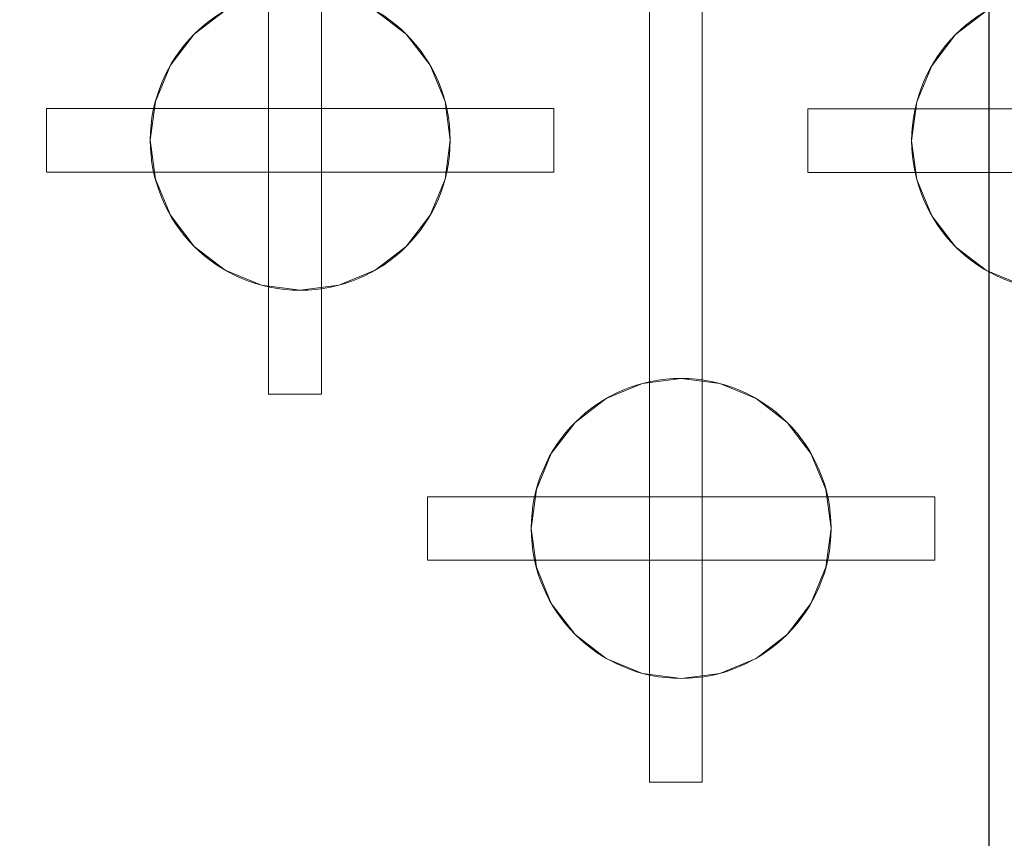
# Model space of a CAD drawing. Units: inches. Extents: x 2696 to 3240, y 1564 to 2310.
# Tile 44 of 76: x 2777.108 to 2782.926, y 2084.368 to 2089.203. Entities that reach past the tile are written whole.
import ezdxf

# ---------------------------------------------------------------- set-up
doc = ezdxf.new("R2010")
doc.units = ezdxf.units.IN
for name, color, linetype, lineweight in [('A-ANNO-DIMS', 3, 'Continuous', 18), ('A-FLOR-FIXT', 8, 'Continuous', 18), ('A-FURN', 251, 'Continuous', 13)]:
    doc.layers.add(name, color=color, linetype=linetype, lineweight=lineweight)
doc.styles.add('TIMES NEW', font='times.ttf')
doc.dimstyles.new('Siddhuu', dxfattribs={"dimtxt": 6, "dimasz": 2.5, "dimexe": 1.25, "dimexo": 0.625, "dimtad": 1, "dimdec": 1, "dimlunit": 4, "dimtxsty": 'TIMES NEW', "dimcen": 2.5, "dimclrd": 256, "dimclre": 1, "dimclrt": 7, "dimadec": 0, "dimazin": 0, "dimtfac": 1, "dimtdec": 1, "dimtmove": 0, "dimatfit": 3, "dimfxl": 1, "dimtolj": 1, "dimlwd": -1, "dimarcsym": 0})

# ---------------------------------------------------------------- blocks, each defined once
blk = doc.blocks.new('A$C1af1f523')
at = {"layer": 'A-FURN'}
for p, q in [((-2.9003, 3.9351), (-2.9003, 0.9365)), ((-2.9003, 3.9351, 0.5), (-2.9003, 0.9365, 0.5)), ((-2.5253, 3.9351), (-2.5253, 0.9365)), ((-2.5253, 3.9351, 0.5), (-2.5253, 0.9365, 0.5)), ((-3.4801, 1.9924), (-3.4801, 1.9924, 0.5)), ((-3.3393, 1.8089), (-3.3393, 1.8089, 0.5)), ((-2.0863, 1.8089), (-2.0863, 1.8089, 0.5)), ((-4.8156, 1.6871), (-5.1906, 1.6871)), ((-4.8156, 1.6871, 0.5), (-5.1906, 1.6871, 0.5)), ((-5.1906, 1.6871), (-5.1906, 1.6871, 0.5)), ((-5.1906, 1.6871), (-5.1901, -1.3115)), ((-5.1906, 1.6871, 0.5), (-5.1901, -1.3115, 0.5)), ((-4.8156, 1.6871), (-4.8156, 1.6871, 0.5)), ((-4.8156, 1.6871), (-4.8151, -1.3115)), ((-4.8156, 1.6871, 0.5), (-4.8151, -1.3115, 0.5)), ((-3.1558, 1.6681), (-3.1558, 1.6681, 0.5)), ((-2.2698, 1.6681), (-2.2698, 1.6681, 0.5)), ((-2.9421, 1.5796), (-2.9421, 1.5796, 0.5)), ((-2.4835, 1.5796), (-2.4835, 1.5796, 0.5)), ((-2.7128, 1.5494), (-2.7128, 1.5494, 0.5)), ((-5.0026, 1.0735), (-5.0026, 1.0735, 0.5)), ((-5.232, 1.0433), (-5.232, 1.0433, 0.5)), ((-4.7733, 1.0433), (-4.7733, 1.0433, 0.5)), ((-5.4457, 0.9548), (-5.4457, 0.9548, 0.5)), ((-4.5596, 0.9548), (-4.5596, 0.9548, 0.5)), ((-2.9003, 0.9365), (-2.9003, 0.9365, 0.5)), ((-2.5253, 0.9365), (-2.8979, 0.9365)), ((-2.5253, 0.9365, 0.5), (-2.8979, 0.9365, 0.5)), ((-2.8979, 0.9365), (-2.8979, 0.9365, 0.5)), ((-2.5253, 0.9365), (-2.5253, 0.9365, 0.5)), ((-5.6292, 0.814), (-5.6292, 0.814, 0.5)), ((-4.3761, 0.814), (-4.3761, 0.814, 0.5)), ((-5.77, 0.6305), (-5.77, 0.6305, 0.5)), ((-4.2353, 0.6305), (-4.2353, 0.6305, 0.5)), ((-5.8585, 0.4168), (-5.8585, 0.4168, 0.5)), ((-4.1468, 0.4168), (-4.1468, 0.4168, 0.5)), ((0, 0.3125), (-6.5015, 0.3125)), ((0, 0.3125, 0.5), (-6.5015, 0.3125, 0.5)), ((-6.5015, 0.3125), (-6.5015, 0.3125, 0.5)), ((-6.5015, 0.3114), (-6.5015, 0)), ((-6.5015, 0.3114, 0.5), (-6.5015, 0, 0.5)), ((-6.5015, 0.3114), (-6.5015, 0.3114, 0.5)), ((-5.8887, 0.1875), (-5.8887, 0.1875, 0.5)), ((-4.1166, 0.1875), (-4.1166, 0.1875, 0.5)), ((0, 0), (-6.5015, 0)), ((0, 0, 0.5), (-6.5015, 0, 0.5)), ((-6.5015, 0), (-6.5015, 0, 0.5)), ((-6.5015, 0), (-6.5015, -0.0011)), ((-6.5015, 0, 0.5), (-6.5015, -0.0011, 0.5)), ((-6.5015, -0.0011), (-6.5015, -0.0011, 0.5)), ((-5.8585, -0.0418), (-5.8585, -0.0418, 0.5)), ((-4.1468, -0.0418), (-4.1468, -0.0418, 0.5)), ((-5.77, -0.2555), (-5.77, -0.2555, 0.5)), ((-4.2353, -0.2555), (-4.2353, -0.2555, 0.5)), ((-5.6292, -0.439), (-5.6292, -0.439, 0.5)), ((-4.3761, -0.439), (-4.3761, -0.439, 0.5)), ((-5.4457, -0.5798), (-5.4457, -0.5798, 0.5)), ((-4.5596, -0.5798), (-4.5596, -0.5798, 0.5)), ((-2.898, -0.5642), (-2.898, -3.5628)), ((-2.898, -0.5642, 0.5), (-2.898, -3.5628, 0.5)), ((-2.898, -0.5642), (-2.898, -0.5642, 0.5)), ((-2.523, -0.5642), (-2.898, -0.5642)), ((-2.523, -0.5642, 0.5), (-2.898, -0.5642, 0.5)), ((-2.523, -0.5642), (-2.523, -3.5628)), ((-2.523, -0.5642, 0.5), (-2.523, -3.5628, 0.5)), ((-2.523, -0.5642), (-2.523, -0.5642, 0.5)), ((-5.232, -0.6683), (-5.232, -0.6683, 0.5)), ((-4.7733, -0.6683), (-4.7733, -0.6683, 0.5)), ((-5.0026, -0.6985), (-5.0026, -0.6985, 0.5)), ((-2.9398, -1.208), (-2.9398, -1.208, 0.5)), ((-2.7105, -1.1778), (-2.7105, -1.1778, 0.5)), ((-2.4812, -1.208), (-2.4812, -1.208, 0.5)), ((-5.1901, -1.3115), (-5.1901, -1.3115, 0.5)), ((-4.8151, -1.3115), (-5.1878, -1.3115)), ((-4.8151, -1.3115, 0.5), (-5.1878, -1.3115, 0.5)), ((-5.1878, -1.3115), (-5.1878, -1.3115, 0.5)), ((-4.8151, -1.3115), (-4.8151, -1.3115, 0.5)), ((-3.1535, -1.2965), (-3.1535, -1.2965, 0.5)), ((-2.2675, -1.2965), (-2.2675, -1.2965, 0.5)), ((-3.337, -1.4373), (-3.337, -1.4373, 0.5)), ((-2.084, -1.4373), (-2.084, -1.4373, 0.5)), ((-3.4778, -1.6208), (-3.4778, -1.6208, 0.5)), ((-3.5664, -1.8345), (-3.5664, -1.8345, 0.5)), ((0, -1.9388), (-4.2094, -1.9388)), ((0, -1.9388, 0.5), (-4.2094, -1.9388, 0.5)), ((-4.2094, -1.9388), (-4.2094, -1.9388, 0.5)), ((-4.2094, -1.9399), (-4.2094, -2.2513)), ((-4.2094, -1.9399, 0.5), (-4.2094, -2.2513, 0.5)), ((-4.2094, -1.9399), (-4.2094, -1.9399, 0.5)), ((-3.5965, -2.0638), (-3.5965, -2.0638, 0.5)), ((0, -2.2513), (-4.2094, -2.2513)), ((0, -2.2513, 0.5), (-4.2094, -2.2513, 0.5)), ((-4.2094, -2.2513), (-4.2094, -2.2513, 0.5)), ((-4.2094, -2.2513), (-4.2094, -2.2524)), ((-4.2094, -2.2513, 0.5), (-4.2094, -2.2524, 0.5)), ((-4.2094, -2.2524), (-4.2094, -2.2524, 0.5)), ((-3.5664, -2.2931), (-3.5664, -2.2931, 0.5)), ((-3.4778, -2.5068), (-3.4778, -2.5068, 0.5)), ((-3.337, -2.6903), (-3.337, -2.6903, 0.5)), ((-2.084, -2.6903), (-2.084, -2.6903, 0.5)), ((-3.1535, -2.8311), (-3.1535, -2.8311, 0.5)), ((-2.2675, -2.8311), (-2.2675, -2.8311, 0.5)), ((-2.9398, -2.9196), (-2.9398, -2.9196, 0.5)), ((-2.7105, -2.9498), (-2.7105, -2.9498, 0.5)), ((-2.4812, -2.9196), (-2.4812, -2.9196, 0.5)), ((-2.898, -3.5628), (-2.898, -3.5628, 0.5)), ((-2.523, -3.5628), (-2.8956, -3.5628)), ((-2.523, -3.5628, 0.5), (-2.8956, -3.5628, 0.5)), ((-2.8956, -3.5628), (-2.8956, -3.5628, 0.5)), ((-2.523, -3.5628), (-2.523, -3.5628, 0.5))]:
    blk.add_line(p, q, dxfattribs=at)
for centre in [(-2.7128, 2.4355), (-2.7128, 2.4355, 0.5), (-5.0026, 0.1875), (-5.0026, 0.1875, 0.5), (-2.7105, -2.0638), (-2.7105, -2.0638, 0.5)]:
    blk.add_circle(centre, 0.886, dxfattribs=at)
mesh = blk.add_polyface(dxfattribs=at)
corners = [(-2.9003, 0.9365, 0.5), (-2.9003, 3.9351), (-2.9003, 0.9365), (-2.9003, 3.9351, 0.5)]
mesh.append_faces([[corners[k] for k in face] for face in [(2, 1, 0), (3, 0, 1)]], dxfattribs={"vtx1": -1})
mesh = blk.add_polyface(dxfattribs=at)
corners = [(-2.5253, 0.9365, 0.5), (-2.5253, 3.9351), (-2.5253, 0.9365), (-2.5253, 3.9351, 0.5)]
mesh.append_faces([[corners[k] for k in face] for face in [(2, 1, 0), (3, 0, 1)]], dxfattribs={"vtx1": -1})
mesh = blk.add_polyface(dxfattribs=at)
corners = [(-3.5686, 2.2061, 0.5), (-3.4801, 1.9924), (-3.5686, 2.2061), (-3.4801, 1.9924, 0.5)]
mesh.append_faces([[corners[k] for k in face] for face in [(2, 1, 0), (3, 0, 1)]], dxfattribs={"vtx1": -1})
mesh = blk.add_polyface(dxfattribs=at)
corners = [(-3.4801, 1.9924, 0.5), (-3.3393, 1.8089), (-3.4801, 1.9924), (-3.3393, 1.8089, 0.5)]
mesh.append_faces([[corners[k] for k in face] for face in [(2, 1, 0), (3, 0, 1)]], dxfattribs={"vtx1": -1})
mesh = blk.add_polyface(dxfattribs=at)
corners = [(-2.0863, 1.8089, 0.5), (-1.9455, 1.9924), (-2.0863, 1.8089), (-1.9455, 1.9924, 0.5)]
mesh.append_faces([[corners[k] for k in face] for face in [(2, 1, 0), (3, 0, 1)]], dxfattribs={"vtx1": -1})
mesh = blk.add_polyface(dxfattribs=at)
corners = [(-3.1558, 1.6681, 0.5), (-3.3393, 1.8089), (-3.3393, 1.8089, 0.5), (-3.1558, 1.6681)]
mesh.append_faces([[corners[k] for k in face] for face in [(2, 1, 0), (3, 0, 1)]], dxfattribs={"vtx1": -1})
mesh = blk.add_polyface(dxfattribs=at)
corners = [(-2.0863, 1.8089, 0.5), (-2.2698, 1.6681), (-2.2698, 1.6681, 0.5), (-2.0863, 1.8089)]
mesh.append_faces([[corners[k] for k in face] for face in [(2, 1, 0), (3, 0, 1)]], dxfattribs={"vtx1": -1})
mesh = blk.add_polyface(dxfattribs=at)
corners = [(-4.8156, 1.6871, 0.5), (-5.1906, 1.6871), (-5.1906, 1.6871, 0.5), (-4.8156, 1.6871)]
mesh.append_faces([[corners[k] for k in face] for face in [(2, 1, 0), (3, 0, 1)]], dxfattribs={"vtx1": -1})
mesh = blk.add_polyface(dxfattribs=at)
corners = [(-5.1901, -1.3115, 0.5), (-5.1906, 1.6871), (-5.1901, -1.3115), (-5.1906, 1.6871, 0.5)]
mesh.append_faces([[corners[k] for k in face] for face in [(2, 1, 0), (3, 0, 1)]], dxfattribs={"vtx1": -1})
mesh = blk.add_polyface(dxfattribs=at)
corners = [(-4.8151, -1.3115, 0.5), (-4.8156, 1.6871), (-4.8151, -1.3115), (-4.8156, 1.6871, 0.5)]
mesh.append_faces([[corners[k] for k in face] for face in [(2, 1, 0), (3, 0, 1)]], dxfattribs={"vtx1": -1})
mesh = blk.add_polyface(dxfattribs=at)
corners = [(-2.9421, 1.5796, 0.5), (-3.1558, 1.6681), (-3.1558, 1.6681, 0.5), (-2.9421, 1.5796)]
mesh.append_faces([[corners[k] for k in face] for face in [(2, 1, 0), (3, 0, 1)]], dxfattribs={"vtx1": -1})
mesh = blk.add_polyface(dxfattribs=at)
corners = [(-2.2698, 1.6681, 0.5), (-2.4835, 1.5796), (-2.4835, 1.5796, 0.5), (-2.2698, 1.6681)]
mesh.append_faces([[corners[k] for k in face] for face in [(2, 1, 0), (3, 0, 1)]], dxfattribs={"vtx1": -1})
mesh = blk.add_polyface(dxfattribs=at)
corners = [(-2.7128, 1.5494, 0.5), (-2.9421, 1.5796), (-2.9421, 1.5796, 0.5), (-2.7128, 1.5494)]
mesh.append_faces([[corners[k] for k in face] for face in [(2, 1, 0), (3, 0, 1)]], dxfattribs={"vtx1": -1})
mesh = blk.add_polyface(dxfattribs=at)
corners = [(-2.4835, 1.5796, 0.5), (-2.7128, 1.5494), (-2.7128, 1.5494, 0.5), (-2.4835, 1.5796)]
mesh.append_faces([[corners[k] for k in face] for face in [(2, 1, 0), (3, 0, 1)]], dxfattribs={"vtx1": -1})
mesh = blk.add_polyface(dxfattribs=at)
corners = [(-5.0026, 1.0735), (-5.232, 1.0433, 0.5), (-5.232, 1.0433), (-5.0026, 1.0735, 0.5)]
mesh.append_faces([[corners[k] for k in face] for face in [(2, 1, 0), (3, 0, 1)]], dxfattribs={"vtx1": -1})
mesh = blk.add_polyface(dxfattribs=at)
corners = [(-4.7733, 1.0433), (-5.0026, 1.0735, 0.5), (-5.0026, 1.0735), (-4.7733, 1.0433, 0.5)]
mesh.append_faces([[corners[k] for k in face] for face in [(2, 1, 0), (3, 0, 1)]], dxfattribs={"vtx1": -1})
mesh = blk.add_polyface(dxfattribs=at)
corners = [(-5.232, 1.0433), (-5.4457, 0.9548, 0.5), (-5.4457, 0.9548), (-5.232, 1.0433, 0.5)]
mesh.append_faces([[corners[k] for k in face] for face in [(2, 1, 0), (3, 0, 1)]], dxfattribs={"vtx1": -1})
mesh = blk.add_polyface(dxfattribs=at)
corners = [(-4.5596, 0.9548), (-4.7733, 1.0433, 0.5), (-4.7733, 1.0433), (-4.5596, 0.9548, 0.5)]
mesh.append_faces([[corners[k] for k in face] for face in [(2, 1, 0), (3, 0, 1)]], dxfattribs={"vtx1": -1})
mesh = blk.add_polyface(dxfattribs=at)
corners = [(-5.4457, 0.9548), (-5.6292, 0.814, 0.5), (-5.6292, 0.814), (-5.4457, 0.9548, 0.5)]
mesh.append_faces([[corners[k] for k in face] for face in [(2, 1, 0), (3, 0, 1)]], dxfattribs={"vtx1": -1})
mesh = blk.add_polyface(dxfattribs=at)
corners = [(-4.3761, 0.814), (-4.5596, 0.9548, 0.5), (-4.5596, 0.9548), (-4.3761, 0.814, 0.5)]
mesh.append_faces([[corners[k] for k in face] for face in [(2, 1, 0), (3, 0, 1)]], dxfattribs={"vtx1": -1})
mesh = blk.add_polyface(dxfattribs=at)
corners = [(-2.5253, 0.9365, 0.5), (-2.8979, 0.9365), (-2.8979, 0.9365, 0.5), (-2.5253, 0.9365)]
mesh.append_faces([[corners[k] for k in face] for face in [(2, 1, 0), (3, 0, 1)]], dxfattribs={"vtx1": -1})
mesh = blk.add_polyface(dxfattribs=at)
corners = [(-5.6292, 0.814, 0.5), (-5.77, 0.6305), (-5.6292, 0.814), (-5.77, 0.6305, 0.5)]
mesh.append_faces([[corners[k] for k in face] for face in [(2, 1, 0), (3, 0, 1)]], dxfattribs={"vtx1": -1})
mesh = blk.add_polyface(dxfattribs=at)
corners = [(-4.2353, 0.6305, 0.5), (-4.3761, 0.814), (-4.2353, 0.6305), (-4.3761, 0.814, 0.5)]
mesh.append_faces([[corners[k] for k in face] for face in [(2, 1, 0), (3, 0, 1)]], dxfattribs={"vtx1": -1})
mesh = blk.add_polyface(dxfattribs=at)
corners = [(-5.77, 0.6305, 0.5), (-5.8585, 0.4168), (-5.77, 0.6305), (-5.8585, 0.4168, 0.5)]
mesh.append_faces([[corners[k] for k in face] for face in [(2, 1, 0), (3, 0, 1)]], dxfattribs={"vtx1": -1})
mesh = blk.add_polyface(dxfattribs=at)
corners = [(-4.1468, 0.4168, 0.5), (-4.2353, 0.6305), (-4.1468, 0.4168), (-4.2353, 0.6305, 0.5)]
mesh.append_faces([[corners[k] for k in face] for face in [(2, 1, 0), (3, 0, 1)]], dxfattribs={"vtx1": -1})
mesh = blk.add_polyface(dxfattribs=at)
corners = [(-5.8585, 0.4168, 0.5), (-5.8887, 0.1875), (-5.8585, 0.4168), (-5.8887, 0.1875, 0.5)]
mesh.append_faces([[corners[k] for k in face] for face in [(2, 1, 0), (3, 0, 1)]], dxfattribs={"vtx1": -1})
mesh = blk.add_polyface(dxfattribs=at)
corners = [(-4.1166, 0.1875, 0.5), (-4.1468, 0.4168), (-4.1166, 0.1875), (-4.1468, 0.4168, 0.5)]
mesh.append_faces([[corners[k] for k in face] for face in [(2, 1, 0), (3, 0, 1)]], dxfattribs={"vtx1": -1})
mesh = blk.add_polyface(dxfattribs=at)
corners = [(0, 0.3125, 0.5), (-6.5015, 0.3125), (-6.5015, 0.3125, 0.5), (0, 0.3125)]
mesh.append_faces([[corners[k] for k in face] for face in [(2, 1, 0), (3, 0, 1)]], dxfattribs={"vtx1": -1})
mesh = blk.add_polyface(dxfattribs=at)
corners = [(-6.5015, -0.0011, 0.5), (-6.5015, 0), (-6.5015, -0.0011), (-6.5015, 0.3114), (-6.5015, 0.3114, 0.5), (-6.5015, 0, 0.5)]
mesh.append_faces([[corners[k] for k in face] for face in [(3, 0, 1), (4, 0, 3)]], dxfattribs={"vtx0": -1, "vtx1": -1})
mesh.append_faces([[corners[k] for k in face] for face in [(2, 1, 0), (5, 0, 4)]], dxfattribs={"vtx1": -1})
mesh = blk.add_polyface(dxfattribs=at)
corners = [(-5.8887, 0.1875, 0.5), (-5.8585, -0.0418), (-5.8887, 0.1875), (-5.8585, -0.0418, 0.5)]
mesh.append_faces([[corners[k] for k in face] for face in [(2, 1, 0), (3, 0, 1)]], dxfattribs={"vtx1": -1})
mesh = blk.add_polyface(dxfattribs=at)
corners = [(-4.1468, -0.0418, 0.5), (-4.1166, 0.1875), (-4.1468, -0.0418), (-4.1166, 0.1875, 0.5)]
mesh.append_faces([[corners[k] for k in face] for face in [(2, 1, 0), (3, 0, 1)]], dxfattribs={"vtx1": -1})
mesh = blk.add_polyface(dxfattribs=at)
corners = [(0, 0, 0.5), (-6.5015, 0), (-6.5015, 0, 0.5), (0, 0)]
mesh.append_faces([[corners[k] for k in face] for face in [(2, 1, 0), (3, 0, 1)]], dxfattribs={"vtx1": -1})
mesh = blk.add_polyface(dxfattribs=at)
corners = [(-5.8585, -0.0418, 0.5), (-5.77, -0.2555), (-5.8585, -0.0418), (-5.77, -0.2555, 0.5)]
mesh.append_faces([[corners[k] for k in face] for face in [(2, 1, 0), (3, 0, 1)]], dxfattribs={"vtx1": -1})
mesh = blk.add_polyface(dxfattribs=at)
corners = [(-4.2353, -0.2555, 0.5), (-4.1468, -0.0418), (-4.2353, -0.2555), (-4.1468, -0.0418, 0.5)]
mesh.append_faces([[corners[k] for k in face] for face in [(2, 1, 0), (3, 0, 1)]], dxfattribs={"vtx1": -1})
mesh = blk.add_polyface(dxfattribs=at)
corners = [(-5.77, -0.2555, 0.5), (-5.6292, -0.439), (-5.77, -0.2555), (-5.6292, -0.439, 0.5)]
mesh.append_faces([[corners[k] for k in face] for face in [(2, 1, 0), (3, 0, 1)]], dxfattribs={"vtx1": -1})
mesh = blk.add_polyface(dxfattribs=at)
corners = [(-4.3761, -0.439, 0.5), (-4.2353, -0.2555), (-4.3761, -0.439), (-4.2353, -0.2555, 0.5)]
mesh.append_faces([[corners[k] for k in face] for face in [(2, 1, 0), (3, 0, 1)]], dxfattribs={"vtx1": -1})
mesh = blk.add_polyface(dxfattribs=at)
corners = [(-5.4457, -0.5798, 0.5), (-5.6292, -0.439), (-5.6292, -0.439, 0.5), (-5.4457, -0.5798)]
mesh.append_faces([[corners[k] for k in face] for face in [(2, 1, 0), (3, 0, 1)]], dxfattribs={"vtx1": -1})
mesh = blk.add_polyface(dxfattribs=at)
corners = [(-4.3761, -0.439, 0.5), (-4.5596, -0.5798), (-4.5596, -0.5798, 0.5), (-4.3761, -0.439)]
mesh.append_faces([[corners[k] for k in face] for face in [(2, 1, 0), (3, 0, 1)]], dxfattribs={"vtx1": -1})
mesh = blk.add_polyface(dxfattribs=at)
corners = [(-5.232, -0.6683, 0.5), (-5.4457, -0.5798), (-5.4457, -0.5798, 0.5), (-5.232, -0.6683)]
mesh.append_faces([[corners[k] for k in face] for face in [(2, 1, 0), (3, 0, 1)]], dxfattribs={"vtx1": -1})
mesh = blk.add_polyface(dxfattribs=at)
corners = [(-4.5596, -0.5798, 0.5), (-4.7733, -0.6683), (-4.7733, -0.6683, 0.5), (-4.5596, -0.5798)]
mesh.append_faces([[corners[k] for k in face] for face in [(2, 1, 0), (3, 0, 1)]], dxfattribs={"vtx1": -1})
mesh = blk.add_polyface(dxfattribs=at)
corners = [(-2.898, -3.5628, 0.5), (-2.898, -0.5642), (-2.898, -3.5628), (-2.898, -0.5642, 0.5)]
mesh.append_faces([[corners[k] for k in face] for face in [(2, 1, 0), (3, 0, 1)]], dxfattribs={"vtx1": -1})
mesh = blk.add_polyface(dxfattribs=at)
corners = [(-2.523, -0.5642, 0.5), (-2.898, -0.5642), (-2.898, -0.5642, 0.5), (-2.523, -0.5642)]
mesh.append_faces([[corners[k] for k in face] for face in [(2, 1, 0), (3, 0, 1)]], dxfattribs={"vtx1": -1})
mesh = blk.add_polyface(dxfattribs=at)
corners = [(-2.523, -3.5628, 0.5), (-2.523, -0.5642), (-2.523, -3.5628), (-2.523, -0.5642, 0.5)]
mesh.append_faces([[corners[k] for k in face] for face in [(2, 1, 0), (3, 0, 1)]], dxfattribs={"vtx1": -1})
mesh = blk.add_polyface(dxfattribs=at)
corners = [(-5.0026, -0.6985, 0.5), (-5.232, -0.6683), (-5.232, -0.6683, 0.5), (-5.0026, -0.6985)]
mesh.append_faces([[corners[k] for k in face] for face in [(2, 1, 0), (3, 0, 1)]], dxfattribs={"vtx1": -1})
mesh = blk.add_polyface(dxfattribs=at)
corners = [(-4.7733, -0.6683, 0.5), (-5.0026, -0.6985), (-5.0026, -0.6985, 0.5), (-4.7733, -0.6683)]
mesh.append_faces([[corners[k] for k in face] for face in [(2, 1, 0), (3, 0, 1)]], dxfattribs={"vtx1": -1})
mesh = blk.add_polyface(dxfattribs=at)
corners = [(-2.9398, -1.208), (-3.1535, -1.2965, 0.5), (-3.1535, -1.2965), (-2.9398, -1.208, 0.5)]
mesh.append_faces([[corners[k] for k in face] for face in [(2, 1, 0), (3, 0, 1)]], dxfattribs={"vtx1": -1})
mesh = blk.add_polyface(dxfattribs=at)
corners = [(-2.7105, -1.1778), (-2.9398, -1.208, 0.5), (-2.9398, -1.208), (-2.7105, -1.1778, 0.5)]
mesh.append_faces([[corners[k] for k in face] for face in [(2, 1, 0), (3, 0, 1)]], dxfattribs={"vtx1": -1})
mesh = blk.add_polyface(dxfattribs=at)
corners = [(-2.4812, -1.208), (-2.7105, -1.1778, 0.5), (-2.7105, -1.1778), (-2.4812, -1.208, 0.5)]
mesh.append_faces([[corners[k] for k in face] for face in [(2, 1, 0), (3, 0, 1)]], dxfattribs={"vtx1": -1})
mesh = blk.add_polyface(dxfattribs=at)
corners = [(-2.2675, -1.2965), (-2.4812, -1.208, 0.5), (-2.4812, -1.208), (-2.2675, -1.2965, 0.5)]
mesh.append_faces([[corners[k] for k in face] for face in [(2, 1, 0), (3, 0, 1)]], dxfattribs={"vtx1": -1})
mesh = blk.add_polyface(dxfattribs=at)
corners = [(-4.8151, -1.3115, 0.5), (-5.1878, -1.3115), (-5.1878, -1.3115, 0.5), (-4.8151, -1.3115)]
mesh.append_faces([[corners[k] for k in face] for face in [(2, 1, 0), (3, 0, 1)]], dxfattribs={"vtx1": -1})
mesh = blk.add_polyface(dxfattribs=at)
corners = [(-3.1535, -1.2965), (-3.337, -1.4373, 0.5), (-3.337, -1.4373), (-3.1535, -1.2965, 0.5)]
mesh.append_faces([[corners[k] for k in face] for face in [(2, 1, 0), (3, 0, 1)]], dxfattribs={"vtx1": -1})
mesh = blk.add_polyface(dxfattribs=at)
corners = [(-2.084, -1.4373), (-2.2675, -1.2965, 0.5), (-2.2675, -1.2965), (-2.084, -1.4373, 0.5)]
mesh.append_faces([[corners[k] for k in face] for face in [(2, 1, 0), (3, 0, 1)]], dxfattribs={"vtx1": -1})
mesh = blk.add_polyface(dxfattribs=at)
corners = [(-3.337, -1.4373, 0.5), (-3.4778, -1.6208), (-3.337, -1.4373), (-3.4778, -1.6208, 0.5)]
mesh.append_faces([[corners[k] for k in face] for face in [(2, 1, 0), (3, 0, 1)]], dxfattribs={"vtx1": -1})
mesh = blk.add_polyface(dxfattribs=at)
corners = [(-1.9432, -1.6208, 0.5), (-2.084, -1.4373), (-1.9432, -1.6208), (-2.084, -1.4373, 0.5)]
mesh.append_faces([[corners[k] for k in face] for face in [(2, 1, 0), (3, 0, 1)]], dxfattribs={"vtx1": -1})
mesh = blk.add_polyface(dxfattribs=at)
corners = [(-3.4778, -1.6208, 0.5), (-3.5664, -1.8345), (-3.4778, -1.6208), (-3.5664, -1.8345, 0.5)]
mesh.append_faces([[corners[k] for k in face] for face in [(2, 1, 0), (3, 0, 1)]], dxfattribs={"vtx1": -1})
mesh = blk.add_polyface(dxfattribs=at)
corners = [(-3.5664, -1.8345, 0.5), (-3.5965, -2.0638), (-3.5664, -1.8345), (-3.5965, -2.0638, 0.5)]
mesh.append_faces([[corners[k] for k in face] for face in [(2, 1, 0), (3, 0, 1)]], dxfattribs={"vtx1": -1})
mesh = blk.add_polyface(dxfattribs=at)
corners = [(0, -1.9388, 0.5), (-4.2094, -1.9388), (-4.2094, -1.9388, 0.5), (0, -1.9388)]
mesh.append_faces([[corners[k] for k in face] for face in [(2, 1, 0), (3, 0, 1)]], dxfattribs={"vtx1": -1})
mesh = blk.add_polyface(dxfattribs=at)
corners = [(-4.2094, -2.2524, 0.5), (-4.2094, -2.2513), (-4.2094, -2.2524), (-4.2094, -1.9399), (-4.2094, -1.9399, 0.5), (-4.2094, -2.2513, 0.5)]
mesh.append_faces([[corners[k] for k in face] for face in [(3, 0, 1), (4, 0, 3)]], dxfattribs={"vtx0": -1, "vtx1": -1})
mesh.append_faces([[corners[k] for k in face] for face in [(2, 1, 0), (5, 0, 4)]], dxfattribs={"vtx1": -1})
mesh = blk.add_polyface(dxfattribs=at)
corners = [(-3.5965, -2.0638, 0.5), (-3.5664, -2.2931), (-3.5965, -2.0638), (-3.5664, -2.2931, 0.5)]
mesh.append_faces([[corners[k] for k in face] for face in [(2, 1, 0), (3, 0, 1)]], dxfattribs={"vtx1": -1})
mesh = blk.add_polyface(dxfattribs=at)
corners = [(0, -2.2513, 0.5), (-4.2094, -2.2513), (-4.2094, -2.2513, 0.5), (0, -2.2513)]
mesh.append_faces([[corners[k] for k in face] for face in [(2, 1, 0), (3, 0, 1)]], dxfattribs={"vtx1": -1})
mesh = blk.add_polyface(dxfattribs=at)
corners = [(-3.5664, -2.2931, 0.5), (-3.4778, -2.5068), (-3.5664, -2.2931), (-3.4778, -2.5068, 0.5)]
mesh.append_faces([[corners[k] for k in face] for face in [(2, 1, 0), (3, 0, 1)]], dxfattribs={"vtx1": -1})
mesh = blk.add_polyface(dxfattribs=at)
corners = [(-3.4778, -2.5068, 0.5), (-3.337, -2.6903), (-3.4778, -2.5068), (-3.337, -2.6903, 0.5)]
mesh.append_faces([[corners[k] for k in face] for face in [(2, 1, 0), (3, 0, 1)]], dxfattribs={"vtx1": -1})
mesh = blk.add_polyface(dxfattribs=at)
corners = [(-2.084, -2.6903, 0.5), (-1.9432, -2.5068), (-2.084, -2.6903), (-1.9432, -2.5068, 0.5)]
mesh.append_faces([[corners[k] for k in face] for face in [(2, 1, 0), (3, 0, 1)]], dxfattribs={"vtx1": -1})
mesh = blk.add_polyface(dxfattribs=at)
corners = [(-3.1535, -2.8311, 0.5), (-3.337, -2.6903), (-3.337, -2.6903, 0.5), (-3.1535, -2.8311)]
mesh.append_faces([[corners[k] for k in face] for face in [(2, 1, 0), (3, 0, 1)]], dxfattribs={"vtx1": -1})
mesh = blk.add_polyface(dxfattribs=at)
corners = [(-2.084, -2.6903, 0.5), (-2.2675, -2.8311), (-2.2675, -2.8311, 0.5), (-2.084, -2.6903)]
mesh.append_faces([[corners[k] for k in face] for face in [(2, 1, 0), (3, 0, 1)]], dxfattribs={"vtx1": -1})
mesh = blk.add_polyface(dxfattribs=at)
corners = [(-2.9398, -2.9196, 0.5), (-3.1535, -2.8311), (-3.1535, -2.8311, 0.5), (-2.9398, -2.9196)]
mesh.append_faces([[corners[k] for k in face] for face in [(2, 1, 0), (3, 0, 1)]], dxfattribs={"vtx1": -1})
mesh = blk.add_polyface(dxfattribs=at)
corners = [(-2.2675, -2.8311, 0.5), (-2.4812, -2.9196), (-2.4812, -2.9196, 0.5), (-2.2675, -2.8311)]
mesh.append_faces([[corners[k] for k in face] for face in [(2, 1, 0), (3, 0, 1)]], dxfattribs={"vtx1": -1})
mesh = blk.add_polyface(dxfattribs=at)
corners = [(-2.7105, -2.9498, 0.5), (-2.9398, -2.9196), (-2.9398, -2.9196, 0.5), (-2.7105, -2.9498)]
mesh.append_faces([[corners[k] for k in face] for face in [(2, 1, 0), (3, 0, 1)]], dxfattribs={"vtx1": -1})
mesh = blk.add_polyface(dxfattribs=at)
corners = [(-2.4812, -2.9196, 0.5), (-2.7105, -2.9498), (-2.7105, -2.9498, 0.5), (-2.4812, -2.9196)]
mesh.append_faces([[corners[k] for k in face] for face in [(2, 1, 0), (3, 0, 1)]], dxfattribs={"vtx1": -1})
mesh = blk.add_polyface(dxfattribs=at)
corners = [(-2.523, -3.5628, 0.5), (-2.8956, -3.5628), (-2.8956, -3.5628, 0.5), (-2.523, -3.5628)]
mesh.append_faces([[corners[k] for k in face] for face in [(2, 1, 0), (3, 0, 1)]], dxfattribs={"vtx1": -1})
blk = doc.blocks.new('*D40')
at = {"layer": 'A-ANNO-DIMS', "color": 1, "lineweight": -2, "transparency": 16777216}
for p, q in [((2777.2662, 2091.8261), (2777.2662, 2093.5758)), ((2784.7641, 2091.8261), (2784.7641, 2093.5758))]:
    blk.add_line(p, q, dxfattribs=at)
at = {"layer": 'A-ANNO-DIMS', "transparency": 16777216}
for p, q in [((2779.7662, 2092.3258), (2782.2641, 2092.3258)), ((2784.7641, 2092.3258), (2902.4579, 2092.3258))]:
    blk.add_line(p, q, dxfattribs=at)
for points in [[(2779.7662, 2092.7424), (2779.7662, 2091.9091), (2777.2662, 2092.3258)], [(2782.2641, 2092.7424), (2782.2641, 2091.9091), (2784.7641, 2092.3258)]]:
    blk.add_solid(points, dxfattribs=at)
at = {"layer": 'Defpoints', "color": 0, "transparency": 16777216}
for p in [(2784.7641, 2092.3258), (2777.2662, 2091.2011), (2784.7641, 2091.2011)]:
    blk.add_point(p, dxfattribs=at)
at = {"layer": 'A-ANNO-DIMS', "color": 7, "transparency": 16777216, "insert": (2844.861, 2096.0935), "char_height": 6, "attachment_point": 5, "style": 'TIMES NEW'}
blk.add_mtext('\\A1;BATH FITTING 0\'-7 1/2" TYP.', dxfattribs=at)
blk = doc.blocks.new('*D41')
at = {"layer": 'A-ANNO-DIMS', "transparency": 16777216}
for p, q in [((2776.1416, 2091.2011), (2776.1416, 2145.7283)), ((2776.1416, 2087.1996), (2776.1416, 2088.7011))]:
    blk.add_line(p, q, dxfattribs=at)
at = {"layer": 'A-ANNO-DIMS', "color": 1, "lineweight": -2, "transparency": 16777216}
for p, q in [((2776.6412, 2091.2011), (2774.8916, 2091.2011)), ((2776.6412, 2084.6996), (2774.8916, 2084.6996))]:
    blk.add_line(p, q, dxfattribs=at)
at = {"layer": 'A-ANNO-DIMS', "transparency": 16777216}
for points in [[(2775.7249, 2088.7011), (2776.5582, 2088.7011), (2776.1416, 2091.2011)], [(2775.7249, 2087.1996), (2776.5582, 2087.1996), (2776.1416, 2084.6996)]]:
    blk.add_solid(points, dxfattribs=at)
at = {"layer": 'Defpoints', "color": 0, "transparency": 16777216}
for p in [(2776.1416, 2091.2011), (2777.2662, 2091.2011), (2777.2662, 2084.6996)]:
    blk.add_point(p, dxfattribs=at)
at = {"layer": 'A-ANNO-DIMS', "color": 7, "transparency": 16777216, "insert": (2772.3803, 2119.7147), "char_height": 6, "attachment_point": 5, "rotation": 90, "style": 'TIMES NEW'}
blk.add_mtext('\\A1;0\'-6 1/2" TYP.', dxfattribs=at)
blk = doc.blocks.new('*D62')
at = {"layer": 'A-ANNO-DIMS', "color": 1, "lineweight": -2, "transparency": 16777216}
for p, q in [((2965.0838, 2140.7011), (2709.3614, 2140.7011)), ((2965.0838, 2063.5906), (2709.3614, 2063.5906))]:
    blk.add_line(p, q, dxfattribs=at)
at = {"layer": 'A-ANNO-DIMS', "transparency": 16777216}
blk.add_line((2710.6114, 2066.0906), (2710.6114, 2138.2011), dxfattribs=at)
for points in [[(2710.1947, 2138.2011), (2711.0281, 2138.2011), (2710.6114, 2140.7011)], [(2710.1947, 2066.0906), (2711.0281, 2066.0906), (2710.6114, 2063.5906)]]:
    blk.add_solid(points, dxfattribs=at)
at = {"layer": 'Defpoints', "color": 0, "transparency": 16777216}
for p in [(2710.6114, 2140.7011), (2965.7088, 2140.7011), (2965.7088, 2063.5906)]:
    blk.add_point(p, dxfattribs=at)
at = {"layer": 'A-ANNO-DIMS', "color": 7, "transparency": 16777216, "insert": (2706.9345, 2102.1459), "char_height": 6, "attachment_point": 5, "rotation": 90, "style": 'TIMES NEW'}
blk.add_mtext('\\A1;6\'-5"', dxfattribs=at)
blk = doc.blocks.new('*D64')
at = {"layer": 'A-ANNO-DIMS', "color": 1, "lineweight": -2, "transparency": 16777216}
for p, q in [((3073.0838, 2206.7011), (2709.3614, 2206.7011)), ((3068.5838, 1989.2011), (2709.3614, 1989.2011))]:
    blk.add_line(p, q, dxfattribs=at)
at = {"layer": 'A-ANNO-DIMS', "transparency": 16777216}
blk.add_line((2710.6114, 1991.7011), (2710.6114, 2204.2011), dxfattribs=at)
for points in [[(2710.1947, 2204.2011), (2711.0281, 2204.2011), (2710.6114, 2206.7011)], [(2710.1947, 1991.7011), (2711.0281, 1991.7011), (2710.6114, 1989.2011)]]:
    blk.add_solid(points, dxfattribs=at)
at = {"layer": 'Defpoints', "color": 0, "transparency": 16777216}
for p in [(2710.6114, 2206.7011), (3073.7088, 2206.7011), (3069.2088, 1989.2011)]:
    blk.add_point(p, dxfattribs=at)
at = {"layer": 'A-ANNO-DIMS', "color": 7, "transparency": 16777216, "insert": (2706.8501, 2097.9511), "char_height": 6, "attachment_point": 5, "rotation": 90, "style": 'TIMES NEW'}
blk.add_mtext('\\A1;18\'-1 1/2"', dxfattribs=at)
blk = doc.blocks.new('*D66')
at = {"layer": 'A-ANNO-DIMS', "color": 1, "lineweight": -2, "transparency": 16777216}
for p, q in [((3077.5838, 2122.7011), (2709.3614, 2122.7011)), ((3077.5838, 2074.7011), (2709.3614, 2074.7011))]:
    blk.add_line(p, q, dxfattribs=at)
at = {"layer": 'A-ANNO-DIMS', "transparency": 16777216}
blk.add_line((2710.6114, 2077.2011), (2710.6114, 2120.2011), dxfattribs=at)
for points in [[(2710.1947, 2120.2011), (2711.0281, 2120.2011), (2710.6114, 2122.7011)], [(2710.1947, 2077.2011), (2711.0281, 2077.2011), (2710.6114, 2074.7011)]]:
    blk.add_solid(points, dxfattribs=at)
at = {"layer": 'Defpoints', "color": 0, "transparency": 16777216}
for p in [(2710.6114, 2122.7011), (3078.2088, 2122.7011), (3078.2088, 2074.7011)]:
    blk.add_point(p, dxfattribs=at)
at = {"layer": 'A-ANNO-DIMS', "color": 7, "transparency": 16777216, "insert": (2706.9345, 2098.7011), "char_height": 6, "attachment_point": 5, "rotation": 90, "style": 'TIMES NEW'}
blk.add_mtext('\\A1;4\'-0"', dxfattribs=at)
blk = doc.blocks.new('*D68')
at = {"layer": 'A-ANNO-DIMS', "color": 1, "lineweight": -2, "transparency": 16777216}
for p, q in [((2745.6114, 2261.5761), (2745.6114, 1568.9511)), ((2782.8338, 2261.5761), (2782.8338, 1568.9511))]:
    blk.add_line(p, q, dxfattribs=at)
at = {"layer": 'A-ANNO-DIMS', "transparency": 16777216}
blk.add_line((2748.1114, 1570.2011), (2780.3338, 1570.2011), dxfattribs=at)
for points in [[(2748.1114, 1570.6178), (2748.1114, 1569.7844), (2745.6114, 1570.2011)], [(2780.3338, 1570.6178), (2780.3338, 1569.7844), (2782.8338, 1570.2011)]]:
    blk.add_solid(points, dxfattribs=at)
at = {"layer": 'Defpoints', "color": 0, "transparency": 16777216}
for p in [(2745.6114, 2262.2011), (2782.8338, 2262.2011), (2782.8338, 1570.2011)]:
    blk.add_point(p, dxfattribs=at)
at = {"layer": 'A-ANNO-DIMS', "color": 7, "transparency": 16777216, "insert": (2764.2226, 1573.878), "char_height": 6, "attachment_point": 5, "style": 'TIMES NEW'}
blk.add_mtext('\\A1;3\'-1"', dxfattribs=at)

msp = doc.modelspace()

# ---------------------------------------------------------------- block references
at = {"layer": 'A-FLOR-FIXT', "xscale": -1, "rotation": 270}
msp.add_blockref('A$C1af1f523', (2780.829, 2091.2011), dxfattribs=at)

# ---------------------------------------------------------------- dimensions: what is measured, and where the dimension line sits
at = {"layer": 'A-ANNO-DIMS'}
dim = msp.add_linear_dim(base=(2782.8338, 1570.2011), p1=(2745.6114, 2262.2011), p2=(2782.8338, 2262.2011), dimstyle='Siddhuu', override={"dimdec": 1, "dimlfac": 1, "dimrnd": 0, "dimzin": 1, "dimdsep": 46, "dimlunit": 4, "dimfrac": 2}, dxfattribs=at)
dim.commit()
dim.dimension.update_dxf_attribs({"geometry": '*D68', "text_midpoint": (2764.2226, 1573.878)})
for base, p1, p2, picture, middle in [((2710.6114, 2206.7011), (3069.2088, 1989.2011), (3073.7088, 2206.7011), '*D64', (2706.8501, 2097.9511)), ((2710.6114, 2140.7011), (2965.7088, 2063.5906), (2965.7088, 2140.7011), '*D62', (2706.9345, 2102.1459)), ((2710.6114, 2122.7011), (3078.2088, 2074.7011), (3078.2088, 2122.7011), '*D66', (2706.9345, 2098.7011))]:
    dim = msp.add_linear_dim(base=base, p1=p1, p2=p2, angle=90, dimstyle='Siddhuu', override={"dimdec": 1, "dimlfac": 1, "dimrnd": 0, "dimzin": 1, "dimdsep": 46, "dimlunit": 4, "dimfrac": 2}, dxfattribs=at)
    dim.commit()
    dim.dimension.update_dxf_attribs({"geometry": picture, "text_midpoint": middle})
dim = msp.add_linear_dim(base=(2776.1416, 2091.2011), p1=(2777.2662, 2084.6996), p2=(2777.2662, 2091.2011), angle=90, text='<> TYP.', dimstyle='Siddhuu', override={"dimdec": 1, "dimlfac": 1, "dimrnd": 0, "dimzin": 1, "dimdsep": 46, "dimlunit": 4, "dimfrac": 2}, dxfattribs=at)
dim.commit()
dim.dimension.update_dxf_attribs({"geometry": '*D41', "text_midpoint": (2772.3803, 2119.7147)})
dim = msp.add_linear_dim(base=(2784.7641, 2092.3258), p1=(2777.2662, 2091.2011), p2=(2784.7641, 2091.2011), text='BATH FITTING <> TYP.', dimstyle='Siddhuu', override={"dimdec": 1, "dimlfac": 1, "dimrnd": 0, "dimzin": 1, "dimdsep": 46, "dimlunit": 4, "dimfrac": 2}, dxfattribs=at)
dim.commit()
dim.dimension.update_dxf_attribs({"geometry": '*D40', "text_midpoint": (2844.861, 2096.0935)})

doc.saveas('drawing.dxf')
